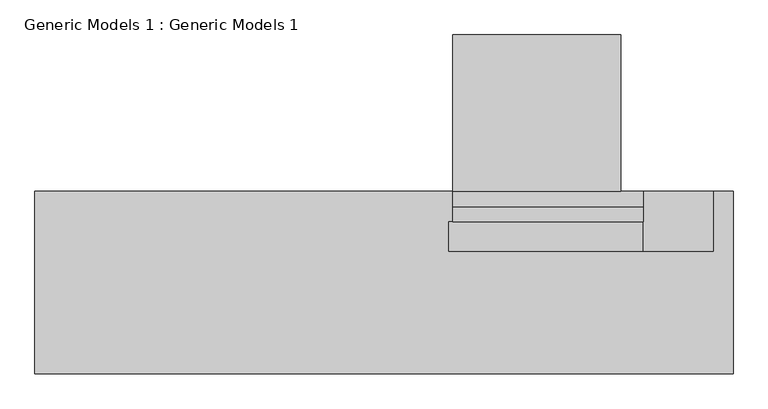
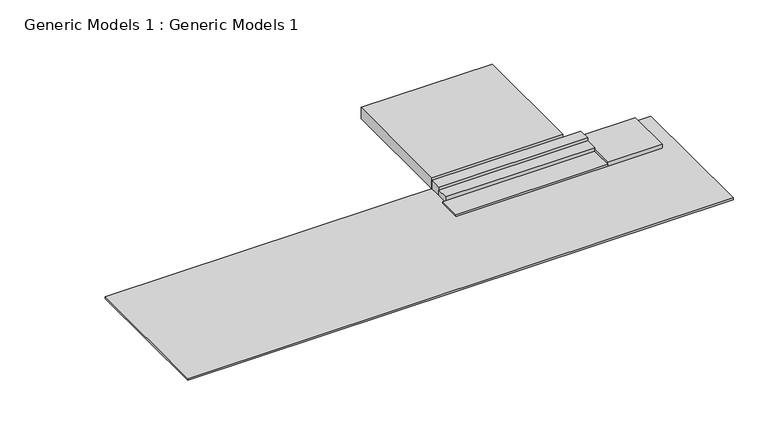
"""IFC4 building model written with IfcOpenShell, lengths in millimetres: proxy geometry, Generic Models 1 : Generic Models 1."""

from ifc_helpers import new_model, si_unit, frame, origin, origin_with_axes, place, context, project, spatial, polyline, outline, extrude, source, transform, mapped, element, save


def generic_models_1_generic_models_1_ed8fc7ec(model_context):
    return source(origin(), model_context, "Body", "SweptSolid", [
        extrude(outline(polyline([(-6368.9831929, -11480.2592534), (-10255.1831929, -11480.2592534), (-10255.1831929, -10896.0592534), (-6368.9831929, -10896.0592534), (-6368.9831929, -11480.2592534)])), frame((0.0, 0.0, -279.4), z_axis=(0.0, 0.0, 1.0), x_axis=(1.0, 0.0, 0.0)), (0.0, 0.0, 1.0), 332.903275),
        extrude(outline(polyline([(-6307.4458891, -11223.6654182), (-10117.4458891, -11223.6654182), (-10117.4458891, -10639.4654182), (-6307.4458891, -10639.4654182), (-6307.4458891, -11223.6654182)])), frame((0.0, 0.0, -279.4), z_axis=(0.0, 0.0, 1.0), x_axis=(1.0, 0.0, 0.0)), (0.0, 0.0, 1.0), 228.6),
        extrude(outline(polyline([(-6368.9831929, -11480.2592534), (-6368.9831929, -10286.4592534), (-4971.9831929, -10286.4592534), (-4971.9831929, -11480.2592534), (-6368.9831929, -11480.2592534)])), origin_with_axes(), (0.0, 0.0, 1.0), 101.6),
        extrude(outline(polyline([(-10178.9831929, -10896.0592534), (-10178.9831929, -10591.2592534), (-6368.9831929, -10591.2592534), (-6368.9831929, -10896.0592534), (-10178.9831929, -10896.0592534)])), origin_with_axes(), (0.0, 0.0, 1.0), 152.4),
        extrude(outline(polyline([(-10178.9831929, -10591.2592534), (-10178.9831929, -10286.4592534), (-6368.9831929, -10286.4592534), (-6368.9831929, -10591.2592534), (-10178.9831929, -10591.2592534)])), origin_with_axes(), (0.0, 0.0, 1.0), 228.6),
        extrude(outline(polyline([(-18522.8831929, -10286.4592534), (-4578.2831929, -10286.4592534), (-4578.2831929, -13927.0589553), (-18522.8831929, -13927.0589553), (-18522.8831929, -10286.4592534)])), frame((0.0, 0.0, -50.8), z_axis=(0.0, 0.0, 1.0), x_axis=(1.0, 0.0, 0.0)), (0.0, 0.0, 1.0), 50.8),
        extrude(outline(polyline([(-6826.1831929, -7162.2592534), (-6826.1831929, -10286.4592534), (-10178.9831929, -10286.4592534), (-10178.9831929, -7162.2592534), (-6826.1831929, -7162.2592534)])), origin_with_axes(), (0.0, 0.0, 1.0), 304.8),
    ])


if __name__ == "__main__":
    model = new_model("IFC4")
    model_context = context("Model", 3, world=origin())
    ifc_project = project(units=[si_unit("LENGTHUNIT", "METRE", prefix="MILLI")], contexts=[model_context])
    site = spatial("IfcSite", under=ifc_project)
    building = spatial("IfcBuilding", under=site)
    placement = place(None, origin())
    generic_models_1_generic_models_1_shape = generic_models_1_generic_models_1_ed8fc7ec(model_context)
    element("IfcBuildingElementProxy", 1, Name="Generic Models 1 : Generic Models 1", ObjectType="Generic Models 1 : Generic Models 1", at=placement, inside=building, context=model_context, shape_type="MappedRepresentation", body=[
        mapped(generic_models_1_generic_models_1_shape, transform((0.0, 0.0, 0.0), x_axis=(1.0, 0.0, 0.0), y_axis=(0.0, 1.0, 0.0), z_axis=(0.0, 0.0, 1.0))),
    ])
    save(model, "model.ifc")
